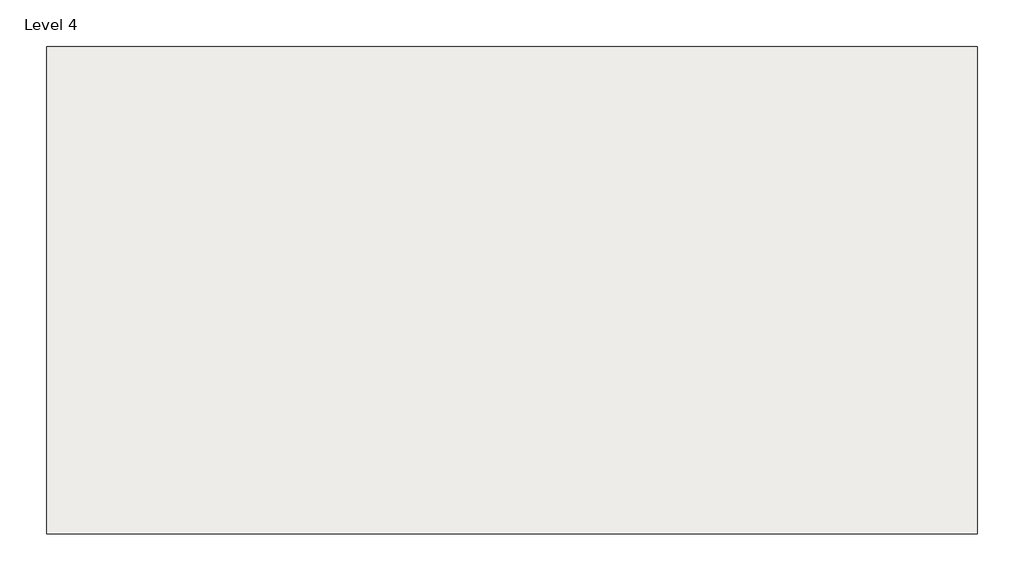
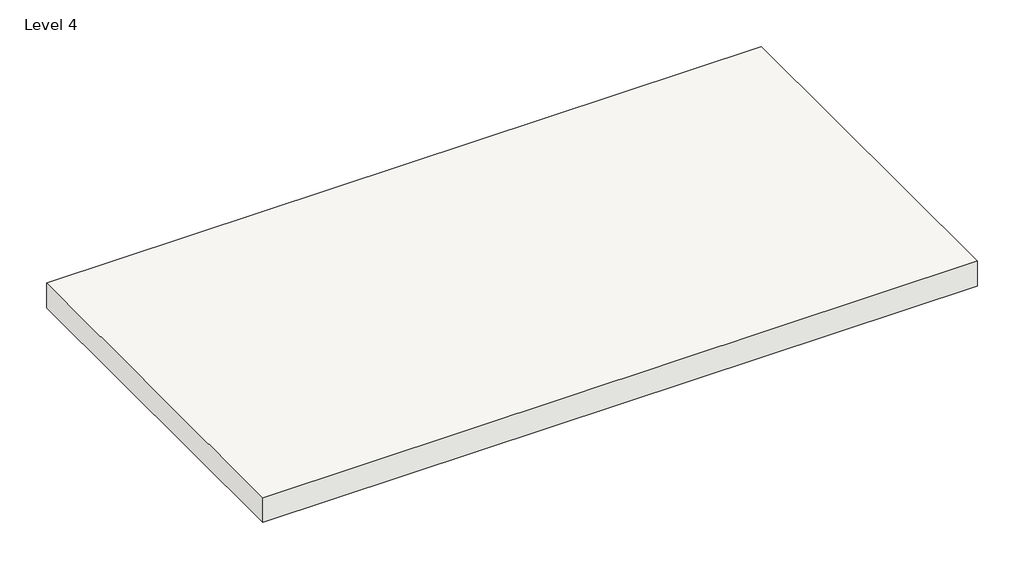
# One storey: 1 roof.
"""IFC4 building model written with IfcOpenShell, lengths in millimetres."""

from ifc_helpers import new_model, si_unit, frame, origin, place, context, project, spatial, polyline, outline, extrude, element, save

model = new_model("IFC4")

# Units and contexts
model_context = context("Model", 3, world=origin())
ifc_project = project(units=[si_unit("LENGTHUNIT", "METRE", prefix="MILLI")], contexts=[model_context])

# Site, building, storey
site = spatial("IfcSite", under=ifc_project)
building = spatial("IfcBuilding", under=site)
storey = spatial("IfcBuildingStorey", under=building, Name="Level 4", Elevation=9144.0)

# Roof
placement = place(None, origin())
element("IfcRoof", 1, ObjectType="Generic - 12\"", at=placement, inside=storey, context=model_context, shape_type="SweptSolid", body=[
    extrude(outline(polyline([(-20474.3003587, -9529.9526331), (-12187.5503587, -9529.9526331), (-12187.5503587, -13873.3526331), (-20474.3003587, -13873.3526331), (-20474.3003587, -9529.9526331)])), frame((0.0, 0.0, 9144.0), z_axis=(0.0, 0.0, 1.0), x_axis=(1.0, 0.0, 0.0)), (0.0, 0.0, 1.0), 304.8),
])

save(model, "model.ifc")

# Revit data of these elements
# Type "Generic - 12\""
#   Assembly Code = "B1020"
#   Layers, outside or top first: 1' - 0" no material (function 1)
# Element 1 (IfcRoof, "Generic - 12\"")
#   built-in parameter 1001705 = 31 (stored number, unit not read)
#   built-in parameter 1001710 = 33615
#   Phase Created = New Construction
#   Materials on its faces: "Default Roof"
# Materials
#   "Default Roof": colour RGB 88 101 114, transparency 0, Cost = 0
